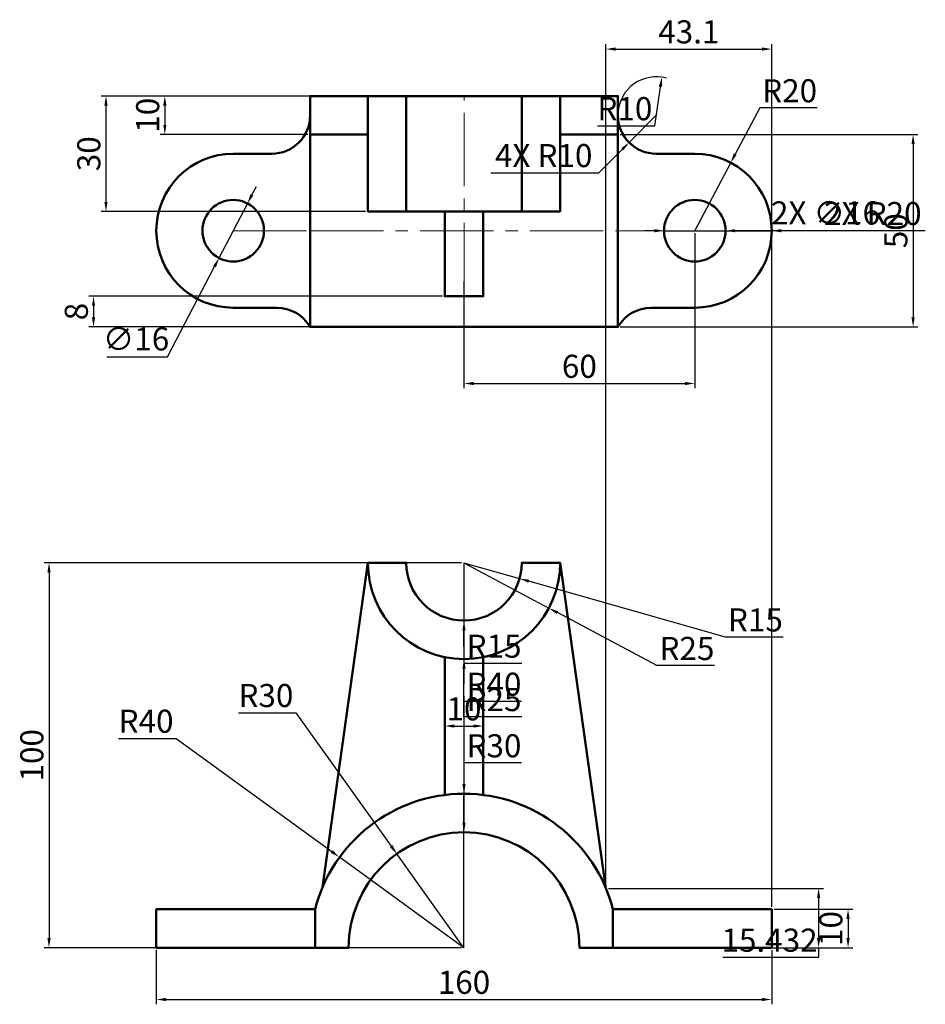
# Model space of a CAD drawing. Units: millimetres. Extents: x 81 to 317, y 95 to 351.
import ezdxf

# ---------------------------------------------------------------- set-up
doc = ezdxf.new("R2010")
doc.units = ezdxf.units.MM
doc.linetypes.add('CENTER2', pattern=[28.575, 19.05, -3.175, 3.175, -3.175])
for name, color, linetype, lineweight in [('M-CNTR', 1, 'CENTER2', 18), ('M-DIMS', 2, 'Continuous', 25), ('M-OUTL', 7, 'Continuous', 50)]:
    doc.layers.add(name, color=color, linetype=linetype, lineweight=lineweight)
doc.styles.get("Standard").update_dxf_attribs({"font": 'arial.ttf'})
doc.dimstyles.new('ISO-25', dxfattribs={"dimtxt": 6, "dimasz": 2.5, "dimexe": 1.25, "dimexo": 0.625, "dimtad": 1, "dimtoh": 1, "dimdec": 0, "dimtxsty": 'Standard', "dimcen": 2.5, "dimadec": 0, "dimazin": 0, "dimtfac": 1, "dimtdec": 0, "dimtmove": 0, "dimatfit": 3, "dimfxl": 1, "dimarcsym": 0})

# ---------------------------------------------------------------- blocks, each defined once
blk = doc.blocks.new('*D1')
at = {"layer": 'Defpoints', "color": 0, "transparency": 16777216}
for p in [(156.66, 331.08), (118.88, 321.08), (156.66, 321.08)]:
    blk.add_point(p, dxfattribs=at)
at = {"layer": 'M-DIMS', "color": 0, "lineweight": -2, "transparency": 16777216}
for p, q in [((156.04, 331.08), (117.63, 331.08)), ((118.88, 328.58), (118.88, 323.58)), ((156.04, 321.08), (117.63, 321.08))]:
    blk.add_line(p, q, dxfattribs=at)
at = {"layer": 'M-DIMS', "color": 0, "transparency": 16777216}
for points in [[(118.47, 328.58), (119.3, 328.58), (118.88, 331.08)], [(118.47, 323.58), (119.3, 323.58), (118.88, 321.08)]]:
    blk.add_solid(points, dxfattribs=at)
at = {"layer": 'M-DIMS', "color": 0, "transparency": 16777216, "insert": (115.2, 326.08), "char_height": 6, "attachment_point": 5, "rotation": 90}
blk.add_mtext('10', dxfattribs=at)
blk = doc.blocks.new('*D2')
at = {"layer": 'Defpoints', "color": 0, "transparency": 16777216}
for p in [(236.66, 321.08), (236.66, 271.08), (313.42, 271.08)]:
    blk.add_point(p, dxfattribs=at)
at = {"layer": 'M-DIMS', "color": 0, "lineweight": -2, "transparency": 16777216}
for p, q in [((237.29, 321.08), (314.67, 321.08)), ((313.42, 318.58), (313.42, 273.58)), ((237.29, 271.08), (314.67, 271.08))]:
    blk.add_line(p, q, dxfattribs=at)
at = {"layer": 'M-DIMS', "color": 0, "transparency": 16777216}
for points in [[(313, 318.58), (313.84, 318.58), (313.42, 321.08)], [(313, 273.58), (313.84, 273.58), (313.42, 271.08)]]:
    blk.add_solid(points, dxfattribs=at)
at = {"layer": 'M-DIMS', "color": 0, "transparency": 16777216, "insert": (309.73, 296.08), "char_height": 6, "attachment_point": 5, "rotation": 90}
blk.add_mtext('50', dxfattribs=at)
blk = doc.blocks.new('*D3')
at = {"layer": 'Defpoints', "color": 0, "transparency": 16777216}
for p in [(171.66, 331.08), (103.58, 301.08), (171.66, 301.08)]:
    blk.add_point(p, dxfattribs=at)
at = {"layer": 'M-DIMS', "color": 0, "lineweight": -2, "transparency": 16777216}
for p, q in [((171.04, 331.08), (102.33, 331.08)), ((103.58, 328.58), (103.58, 303.58)), ((171.04, 301.08), (102.33, 301.08))]:
    blk.add_line(p, q, dxfattribs=at)
at = {"layer": 'M-DIMS', "color": 0, "transparency": 16777216}
for points in [[(103.16, 328.58), (104, 328.58), (103.58, 331.08)], [(103.16, 303.58), (104, 303.58), (103.58, 301.08)]]:
    blk.add_solid(points, dxfattribs=at)
at = {"layer": 'M-DIMS', "color": 0, "transparency": 16777216, "insert": (99.89, 316.08), "char_height": 6, "attachment_point": 5, "rotation": 90}
blk.add_mtext('30', dxfattribs=at)
blk = doc.blocks.new('*D4')
at = {"layer": 'Defpoints', "color": 0, "transparency": 16777216}
for p in [(256.66, 296.08), (196.66, 283.5), (256.66, 256.39)]:
    blk.add_point(p, dxfattribs=at)
at = {"layer": 'M-DIMS', "color": 0, "lineweight": -2, "transparency": 16777216}
for p, q in [((256.66, 295.45), (256.66, 255.14)), ((196.66, 282.87), (196.66, 255.14)), ((199.16, 256.39), (254.16, 256.39))]:
    blk.add_line(p, q, dxfattribs=at)
at = {"layer": 'M-DIMS', "color": 0, "transparency": 16777216}
for points in [[(199.16, 256.81), (199.16, 255.98), (196.66, 256.39)], [(254.16, 256.81), (254.16, 255.98), (256.66, 256.39)]]:
    blk.add_solid(points, dxfattribs=at)
at = {"layer": 'M-DIMS', "color": 0, "transparency": 16777216, "insert": (226.66, 260.08), "char_height": 6, "attachment_point": 5}
blk.add_mtext('60', dxfattribs=at)
blk = doc.blocks.new('*D5')
at = {"layer": 'Defpoints', "color": 0, "transparency": 16777216}
for p in [(191.66, 279.08), (100.34, 271.08), (191.66, 271.08)]:
    blk.add_point(p, dxfattribs=at)
at = {"layer": 'M-DIMS', "color": 0, "lineweight": -2, "transparency": 16777216}
for p, q in [((191.04, 279.08), (99.09, 279.08)), ((100.34, 276.58), (100.34, 273.58)), ((191.04, 271.08), (99.09, 271.08))]:
    blk.add_line(p, q, dxfattribs=at)
at = {"layer": 'M-DIMS', "color": 0, "transparency": 16777216}
for points in [[(99.92, 276.58), (100.75, 276.58), (100.34, 279.08)], [(99.92, 273.58), (100.75, 273.58), (100.34, 271.08)]]:
    blk.add_solid(points, dxfattribs=at)
at = {"layer": 'M-DIMS', "color": 0, "transparency": 16777216, "insert": (96.65, 275.08), "char_height": 6, "attachment_point": 5, "rotation": 90}
blk.add_mtext('8', dxfattribs=at)
blk = doc.blocks.new('*D6')
at = {"layer": 'Defpoints', "color": 0, "transparency": 16777216}
for p in [(266.02, 313.76), (256.66, 296.08)]:
    blk.add_point(p, dxfattribs=at)
at = {"layer": 'M-DIMS', "color": 0, "lineweight": -2, "transparency": 16777216}
for p, q in [((273.54, 327.98), (267.19, 315.97)), ((288.48, 327.98), (273.54, 327.98)), ((256.66, 296.08), (266.02, 313.76))]:
    blk.add_line(p, q, dxfattribs=at)
at = {"layer": 'M-DIMS', "color": 0, "transparency": 16777216}
blk.add_solid([(266.82, 316.16), (267.55, 315.77), (266.02, 313.76)], dxfattribs=at)
at = {"layer": 'M-DIMS', "color": 0, "transparency": 16777216, "insert": (281.32, 331.67), "char_height": 6, "attachment_point": 5}
blk.add_mtext('R20', dxfattribs=at)
blk = doc.blocks.new('*D7')
at = {"layer": 'Defpoints', "color": 0, "transparency": 16777216}
for p in [(140.37, 303.17), (132.96, 288.99)]:
    blk.add_point(p, dxfattribs=at)
at = {"layer": 'M-DIMS', "color": 0, "lineweight": -2, "transparency": 16777216}
for p, q in [((141.52, 305.39), (142.68, 307.6)), ((140.37, 303.17), (132.96, 288.99)), ((119.58, 263.34), (131.81, 286.77)), ((103.84, 263.34), (119.58, 263.34))]:
    blk.add_line(p, q, dxfattribs=at)
at = {"layer": 'M-DIMS', "color": 0, "transparency": 16777216}
for points in [[(141.15, 305.58), (141.89, 305.19), (140.37, 303.17)], [(131.44, 286.96), (132.18, 286.58), (132.96, 288.99)]]:
    blk.add_solid(points, dxfattribs=at)
at = {"layer": 'M-DIMS', "color": 0, "transparency": 16777216, "insert": (111.4, 267.2), "char_height": 6, "attachment_point": 5}
blk.add_mtext('∅16', dxfattribs=at)
blk = doc.blocks.new('*D8')
at = {"layer": 'Defpoints', "color": 0, "transparency": 16777216}
for p in [(248.09, 335.98), (246.66, 326.08)]:
    blk.add_point(p, dxfattribs=at)
at = {"layer": 'M-DIMS', "color": 0, "lineweight": -2, "transparency": 16777216}
for p, q in [((246.27, 323.32), (247.73, 333.5)), ((231.33, 323.32), (246.27, 323.32))]:
    blk.add_line(p, q, dxfattribs=at)
blk.add_arc((246.66, 326.08), 10, 74.6697, 176.419, dxfattribs=at)
at = {"layer": 'M-DIMS', "color": 0, "transparency": 16777216}
blk.add_solid([(247.32, 333.56), (248.14, 333.44), (248.09, 335.98)], dxfattribs=at)
at = {"layer": 'M-DIMS', "color": 0, "transparency": 16777216, "insert": (238.49, 327.01), "char_height": 6, "attachment_point": 5}
blk.add_mtext('R10', dxfattribs=at)
blk = doc.blocks.new('*D9')
at = {"layer": 'Defpoints', "color": 0, "transparency": 16777216}
for p in [(196.66, 209.81), (88.77, 109.81), (196.66, 109.81)]:
    blk.add_point(p, dxfattribs=at)
at = {"layer": 'M-DIMS', "color": 0, "lineweight": -2, "transparency": 16777216}
for p, q in [((196.04, 209.81), (87.52, 209.81)), ((88.77, 207.31), (88.77, 112.31)), ((196.04, 109.81), (87.52, 109.81))]:
    blk.add_line(p, q, dxfattribs=at)
at = {"layer": 'M-DIMS', "color": 0, "transparency": 16777216}
for points in [[(88.35, 207.31), (89.19, 207.31), (88.77, 209.81)], [(88.35, 112.31), (89.19, 112.31), (88.77, 109.81)]]:
    blk.add_solid(points, dxfattribs=at)
at = {"layer": 'M-DIMS', "color": 0, "transparency": 16777216, "insert": (85.08, 159.81), "char_height": 6, "attachment_point": 5, "rotation": 90}
blk.add_mtext('100', dxfattribs=at)
blk = doc.blocks.new('*D10')
at = {"layer": 'Defpoints', "color": 0, "transparency": 16777216}
for p in [(191.66, 167.4), (201.66, 167.4), (201.66, 167.4)]:
    blk.add_point(p, dxfattribs=at)
at = {"layer": 'M-DIMS', "color": 0, "lineweight": -2, "transparency": 16777216}
for p, q in [((191.66, 168.03), (191.66, 168.65)), ((194.16, 167.4), (199.16, 167.4)), ((201.66, 168.03), (201.66, 168.65))]:
    blk.add_line(p, q, dxfattribs=at)
at = {"layer": 'M-DIMS', "color": 0, "transparency": 16777216}
for points in [[(194.16, 167.82), (194.16, 166.99), (191.66, 167.4)], [(199.16, 167.82), (199.16, 166.99), (201.66, 167.4)]]:
    blk.add_solid(points, dxfattribs=at)
at = {"layer": 'M-DIMS', "color": 0, "transparency": 16777216, "insert": (196.66, 171.09), "char_height": 6, "attachment_point": 5}
blk.add_mtext('10', dxfattribs=at)
blk = doc.blocks.new('*D11')
at = {"layer": 'Defpoints', "color": 0, "transparency": 16777216}
for p in [(276.66, 119.81), (276.66, 109.81), (296.51, 109.81)]:
    blk.add_point(p, dxfattribs=at)
at = {"layer": 'M-DIMS', "color": 0, "lineweight": -2, "transparency": 16777216}
for p, q in [((277.29, 119.81), (297.76, 119.81)), ((296.51, 117.31), (296.51, 112.31)), ((277.29, 109.81), (297.76, 109.81))]:
    blk.add_line(p, q, dxfattribs=at)
at = {"layer": 'M-DIMS', "color": 0, "transparency": 16777216}
for points in [[(296.09, 117.31), (296.93, 117.31), (296.51, 119.81)], [(296.09, 112.31), (296.93, 112.31), (296.51, 109.81)]]:
    blk.add_solid(points, dxfattribs=at)
at = {"layer": 'M-DIMS', "color": 0, "transparency": 16777216, "insert": (292.82, 114.81), "char_height": 6, "attachment_point": 5, "rotation": 90}
blk.add_mtext('10', dxfattribs=at)
blk = doc.blocks.new('*D12')
at = {"layer": 'Defpoints', "color": 0, "transparency": 16777216}
for p in [(196.66, 209.81), (218.73, 198.05)]:
    blk.add_point(p, dxfattribs=at)
at = {"layer": 'M-DIMS', "color": 0, "lineweight": -2, "transparency": 16777216}
for p, q in [((196.66, 209.81), (218.73, 198.05)), ((246.8, 183.1), (220.94, 196.88)), ((261.81, 183.1), (246.8, 183.1))]:
    blk.add_line(p, q, dxfattribs=at)
at = {"layer": 'M-DIMS', "color": 0, "transparency": 16777216}
blk.add_solid([(221.13, 197.25), (220.74, 196.51), (218.73, 198.05)], dxfattribs=at)
at = {"layer": 'M-DIMS', "color": 0, "transparency": 16777216, "insert": (254.62, 186.79), "char_height": 6, "attachment_point": 5}
blk.add_mtext('R25', dxfattribs=at)
blk = doc.blocks.new('*D13')
at = {"layer": 'Defpoints', "color": 0, "transparency": 16777216}
for p in [(196.66, 209.81), (211.09, 205.71)]:
    blk.add_point(p, dxfattribs=at)
at = {"layer": 'M-DIMS', "color": 0, "lineweight": -2, "transparency": 16777216}
for p, q in [((196.66, 209.81), (211.09, 205.71)), ((264.61, 190.51), (213.5, 205.03)), ((279.61, 190.51), (264.61, 190.51))]:
    blk.add_line(p, q, dxfattribs=at)
at = {"layer": 'M-DIMS', "color": 0, "transparency": 16777216}
blk.add_solid([(213.61, 205.43), (213.39, 204.63), (211.09, 205.71)], dxfattribs=at)
at = {"layer": 'M-DIMS', "color": 0, "transparency": 16777216, "insert": (272.42, 194.2), "char_height": 6, "attachment_point": 5}
blk.add_mtext('R15', dxfattribs=at)
blk = doc.blocks.new('*D14')
at = {"layer": 'Defpoints', "color": 0, "transparency": 16777216}
for p in [(116.66, 109.81), (276.66, 109.81), (276.66, 96.36)]:
    blk.add_point(p, dxfattribs=at)
at = {"layer": 'M-DIMS', "color": 0, "lineweight": -2, "transparency": 16777216}
for p, q in [((116.66, 109.18), (116.66, 95.11)), ((276.66, 109.18), (276.66, 95.11)), ((119.16, 96.36), (274.16, 96.36))]:
    blk.add_line(p, q, dxfattribs=at)
at = {"layer": 'M-DIMS', "color": 0, "transparency": 16777216}
for points in [[(119.16, 96.78), (119.16, 95.95), (116.66, 96.36)], [(274.16, 96.78), (274.16, 95.95), (276.66, 96.36)]]:
    blk.add_solid(points, dxfattribs=at)
at = {"layer": 'M-DIMS', "color": 0, "transparency": 16777216, "insert": (196.66, 100.05), "char_height": 6, "attachment_point": 5}
blk.add_mtext('160', dxfattribs=at)
blk = doc.blocks.new('*D15')
at = {"layer": 'Defpoints', "color": 0, "transparency": 16777216}
for p in [(164.3, 133.32), (196.66, 109.81)]:
    blk.add_point(p, dxfattribs=at)
at = {"layer": 'M-DIMS', "color": 0, "lineweight": -2, "transparency": 16777216}
for p, q in [((106.84, 164.2), (121.79, 164.2)), ((121.79, 164.2), (162.28, 134.79)), ((196.66, 109.81), (164.3, 133.32))]:
    blk.add_line(p, q, dxfattribs=at)
at = {"layer": 'M-DIMS', "color": 0, "transparency": 16777216}
blk.add_solid([(162.52, 135.12), (162.03, 134.45), (164.3, 133.32)], dxfattribs=at)
at = {"layer": 'M-DIMS', "color": 0, "transparency": 16777216, "insert": (114, 167.88), "char_height": 6, "attachment_point": 5}
blk.add_mtext('R40', dxfattribs=at)
blk = doc.blocks.new('*D16')
at = {"layer": 'Defpoints', "color": 0, "transparency": 16777216}
for p in [(179.2, 134.2), (196.66, 109.81)]:
    blk.add_point(p, dxfattribs=at)
at = {"layer": 'M-DIMS', "color": 0, "lineweight": -2, "transparency": 16777216}
for p, q in [((138, 170.87), (152.95, 170.87)), ((152.95, 170.87), (177.74, 136.23)), ((196.66, 109.81), (179.2, 134.2))]:
    blk.add_line(p, q, dxfattribs=at)
at = {"layer": 'M-DIMS', "color": 0, "transparency": 16777216}
blk.add_solid([(178.08, 136.48), (177.41, 135.99), (179.2, 134.2)], dxfattribs=at)
at = {"layer": 'M-DIMS', "color": 0, "transparency": 16777216, "insert": (145.16, 174.56), "char_height": 6, "attachment_point": 5}
blk.add_mtext('R30', dxfattribs=at)
blk = doc.blocks.new('*D17')
at = {"layer": 'Defpoints', "color": 0, "transparency": 16777216}
for p in [(276.66, 343.28), (233.57, 125.24), (276.66, 119.81)]:
    blk.add_point(p, dxfattribs=at)
at = {"layer": 'M-DIMS', "color": 0, "lineweight": -2, "transparency": 16777216}
for p, q in [((233.57, 125.87), (233.57, 344.53)), ((236.07, 343.28), (274.16, 343.28)), ((276.66, 120.43), (276.66, 344.53))]:
    blk.add_line(p, q, dxfattribs=at)
at = {"layer": 'M-DIMS', "color": 0, "transparency": 16777216}
for points in [[(236.07, 343.7), (236.07, 342.86), (233.57, 343.28)], [(274.16, 343.7), (274.16, 342.86), (276.66, 343.28)]]:
    blk.add_solid(points, dxfattribs=at)
at = {"layer": 'M-DIMS', "color": 0, "transparency": 16777216, "insert": (255.12, 346.97), "char_height": 6, "attachment_point": 5}
blk.add_mtext('43.1', dxfattribs=at)
blk = doc.blocks.new('*D18')
at = {"layer": 'Defpoints', "color": 0, "transparency": 16777216}
for p in [(233.57, 125.24), (235.39, 109.81), (288.86, 109.81)]:
    blk.add_point(p, dxfattribs=at)
at = {"layer": 'M-DIMS', "color": 0, "lineweight": -2, "transparency": 16777216}
for p, q in [((234.19, 125.24), (290.11, 125.24)), ((288.86, 122.74), (288.86, 112.31)), ((236.02, 109.81), (290.11, 109.81)), ((288.86, 109.81), (288.86, 107.31)), ((288.86, 107.31), (263.96, 107.31))]:
    blk.add_line(p, q, dxfattribs=at)
at = {"layer": 'M-DIMS', "color": 0, "transparency": 16777216}
for points in [[(288.45, 122.74), (289.28, 122.74), (288.86, 125.24)], [(288.45, 112.31), (289.28, 112.31), (288.86, 109.81)]]:
    blk.add_solid(points, dxfattribs=at)
at = {"layer": 'M-DIMS', "color": 0, "transparency": 16777216, "insert": (276.1, 111), "char_height": 6, "attachment_point": 5}
blk.add_mtext('15.432', dxfattribs=at)
blk = doc.blocks.new('*D19')
at = {"layer": 'Defpoints', "color": 0, "transparency": 16777216}
for p in [(196.66, 149.81), (196.66, 109.81)]:
    blk.add_point(p, dxfattribs=at)
at = {"layer": 'M-DIMS', "color": 0, "lineweight": -2, "transparency": 16777216}
for p, q in [((211.61, 173.81), (196.66, 173.81)), ((196.66, 173.81), (196.66, 152.31)), ((196.66, 109.81), (196.66, 149.81))]:
    blk.add_line(p, q, dxfattribs=at)
at = {"layer": 'M-DIMS', "color": 0, "transparency": 16777216}
blk.add_solid([(196.25, 152.31), (197.08, 152.31), (196.66, 149.81)], dxfattribs=at)
at = {"layer": 'M-DIMS', "color": 0, "transparency": 16777216, "insert": (204.45, 177.5), "char_height": 6, "attachment_point": 5}
blk.add_mtext('R40', dxfattribs=at)
blk = doc.blocks.new('*D20')
at = {"layer": 'Defpoints', "color": 0, "transparency": 16777216}
for p in [(196.66, 139.81), (196.66, 109.81)]:
    blk.add_point(p, dxfattribs=at)
at = {"layer": 'M-DIMS', "color": 0, "lineweight": -2, "transparency": 16777216}
for p, q in [((211.61, 157.81), (196.66, 157.81)), ((196.66, 157.81), (196.66, 142.31)), ((196.66, 109.81), (196.66, 139.81))]:
    blk.add_line(p, q, dxfattribs=at)
at = {"layer": 'M-DIMS', "color": 0, "transparency": 16777216}
blk.add_solid([(196.25, 142.31), (197.08, 142.31), (196.66, 139.81)], dxfattribs=at)
at = {"layer": 'M-DIMS', "color": 0, "transparency": 16777216, "insert": (204.45, 161.5), "char_height": 6, "attachment_point": 5}
blk.add_mtext('R30', dxfattribs=at)
blk = doc.blocks.new('*D21')
at = {"layer": 'Defpoints', "color": 0, "transparency": 16777216}
for p in [(196.66, 209.81), (196.66, 184.81)]:
    blk.add_point(p, dxfattribs=at)
at = {"layer": 'M-DIMS', "color": 0, "lineweight": -2, "transparency": 16777216}
for p, q in [((196.66, 209.81), (196.66, 184.81)), ((196.66, 169.81), (196.66, 182.31)), ((211.67, 169.81), (196.66, 169.81))]:
    blk.add_line(p, q, dxfattribs=at)
at = {"layer": 'M-DIMS', "color": 0, "transparency": 16777216}
blk.add_solid([(197.08, 182.31), (196.25, 182.31), (196.66, 184.81)], dxfattribs=at)
at = {"layer": 'M-DIMS', "color": 0, "transparency": 16777216, "insert": (204.48, 173.5), "char_height": 6, "attachment_point": 5}
blk.add_mtext('R25', dxfattribs=at)
blk = doc.blocks.new('*D22')
at = {"layer": 'Defpoints', "color": 0, "transparency": 16777216}
for p in [(196.66, 209.81), (196.66, 194.81)]:
    blk.add_point(p, dxfattribs=at)
at = {"layer": 'M-DIMS', "color": 0, "lineweight": -2, "transparency": 16777216}
for p, q in [((196.66, 209.81), (196.66, 194.81)), ((196.67, 183.68), (196.66, 192.31)), ((211.67, 183.68), (196.67, 183.68))]:
    blk.add_line(p, q, dxfattribs=at)
at = {"layer": 'M-DIMS', "color": 0, "transparency": 16777216}
blk.add_solid([(197.08, 192.31), (196.25, 192.31), (196.66, 194.81)], dxfattribs=at)
at = {"layer": 'M-DIMS', "color": 0, "transparency": 16777216, "insert": (204.48, 187.37), "char_height": 6, "attachment_point": 5}
blk.add_mtext('R15', dxfattribs=at)
blk = doc.blocks.new('*D23')
at = {"layer": 'Defpoints', "color": 0, "transparency": 16777216}
for p in [(256.66, 296.08), (276.66, 296.08)]:
    blk.add_point(p, dxfattribs=at)
at = {"layer": 'M-DIMS', "color": 0, "lineweight": -2, "transparency": 16777216}
for p, q in [((256.66, 296.08), (276.66, 296.08)), ((288.66, 296.08), (279.16, 296.08)), ((316.6, 296.08), (288.66, 296.08))]:
    blk.add_line(p, q, dxfattribs=at)
at = {"layer": 'M-DIMS', "color": 0, "transparency": 16777216}
blk.add_solid([(279.16, 296.5), (279.16, 295.66), (276.66, 296.08)], dxfattribs=at)
at = {"layer": 'M-DIMS', "color": 0, "transparency": 16777216, "insert": (302.95, 299.77), "char_height": 6, "attachment_point": 5}
blk.add_mtext('2X R20', dxfattribs=at)
blk = doc.blocks.new('*D24')
at = {"layer": 'Defpoints', "color": 0, "transparency": 16777216}
for p in [(246.66, 326.08), (239.59, 319.01)]:
    blk.add_point(p, dxfattribs=at)
at = {"layer": 'M-DIMS', "color": 0, "lineweight": -2, "transparency": 16777216}
for p, q in [((246.66, 326.08), (239.59, 319.01)), ((231.73, 311.14), (237.83, 317.24)), ((203.65, 311.14), (231.73, 311.14))]:
    blk.add_line(p, q, dxfattribs=at)
at = {"layer": 'M-DIMS', "color": 0, "transparency": 16777216}
blk.add_solid([(237.53, 317.53), (238.12, 316.95), (239.59, 319.01)], dxfattribs=at)
at = {"layer": 'M-DIMS', "color": 0, "transparency": 16777216, "insert": (217.38, 314.83), "char_height": 6, "attachment_point": 5}
blk.add_mtext('4X R10', dxfattribs=at)
blk = doc.blocks.new('*D25')
at = {"layer": 'Defpoints', "color": 0, "transparency": 16777216}
for p in [(248.66, 296.08), (264.66, 296.08)]:
    blk.add_point(p, dxfattribs=at)
at = {"layer": 'M-DIMS', "color": 0, "lineweight": -2, "transparency": 16777216}
for p, q in [((246.16, 296.08), (243.66, 296.08)), ((248.66, 296.08), (264.66, 296.08)), ((276.13, 296.08), (267.16, 296.08)), ((304.55, 296.08), (276.13, 296.08))]:
    blk.add_line(p, q, dxfattribs=at)
at = {"layer": 'M-DIMS', "color": 0, "transparency": 16777216}
for points in [[(246.16, 296.5), (246.16, 295.66), (248.66, 296.08)], [(267.16, 296.5), (267.16, 295.66), (264.66, 296.08)]]:
    blk.add_solid(points, dxfattribs=at)
at = {"layer": 'M-DIMS', "color": 0, "transparency": 16777216, "insert": (290.65, 299.94), "char_height": 6, "attachment_point": 5}
blk.add_mtext('2X ∅16', dxfattribs=at)

msp = doc.modelspace()

# ---------------------------------------------------------------- linework, layer by layer
at = {"layer": 'M-CNTR'}
for p, q in [((196.6648, 279.0792), (196.6648, 331.0792)), ((196.6648, 149.8091), (196.6648, 184.8091))]:
    msp.add_line(p, q, dxfattribs=at)
msp.add_lwpolyline([(136.6648, 296.0792), (156.6648, 296.0792), (236.6648, 296.0792), (256.6648, 296.0792)], dxfattribs=at)
at = {"layer": 'M-OUTL'}
for p, q in [((181.6648, 301.0792), (181.6648, 331.0792)), ((211.6648, 301.0792), (211.6648, 331.0792)), ((156.6648, 321.0792), (171.6648, 321.0792)), ((221.6648, 321.0792), (236.6648, 321.0792)), ((236.6648, 271.0792), (156.6648, 271.0792)), ((191.6648, 149.4954), (191.6648, 185.3142)), ((201.6648, 149.4954), (201.6648, 185.3142))]:
    msp.add_line(p, q, dxfattribs=at)
for points in [[(236.6648, 326.0792, 0.41421356), (246.6648, 316.0792), (256.6648, 316.0792, -1), (256.6648, 276.0792), (245.3251, 276.0792, 0.26794919), (236.6648, 271.0792), (236.6648, 324.0792), (236.6648, 331.0792), (156.6648, 331.0792), (156.6648, 271.0792, 0.26794919), (148.0046, 276.0792), (136.6648, 276.0792, -1), (136.6648, 316.0792), (146.6648, 316.0792, 0.41421356), (156.6648, 326.0792)], [(159.8858, 125.535), (171.6648, 209.8091), (181.6648, 209.8091, 1), (211.6648, 209.8091), (221.6648, 209.8091), (233.5681, 125.2412)], [(157.935, 109.8091), (157.935, 119.8091), (116.6648, 119.8091), (116.6648, 109.8091), (156.6648, 109.8091), (166.6648, 109.8091, -1), (226.6648, 109.8091), (236.6648, 109.8091), (276.6648, 109.8091), (276.6648, 119.8091), (235.3946, 119.8091), (235.3946, 109.8091)]]:
    msp.add_lwpolyline(points, format="xyb", dxfattribs=at)
for points in [[(171.6648, 331.0792), (171.6648, 301.0792), (221.6648, 301.0792), (221.6648, 331.0792)], [(201.6648, 301.0792), (201.6648, 279.0792), (191.6648, 279.0792), (191.6648, 301.0792)]]:
    msp.add_lwpolyline(points, dxfattribs=at)
for centre in [(136.6648, 296.0792), (256.6648, 296.0792)]:
    msp.add_circle(centre, 8, dxfattribs=at)
for centre, radius, start, end in [((196.6648, 209.8091), 25, 180, 0), ((196.6648, 109.8091), 40, 14.477512, 165.522488)]:
    msp.add_arc(centre, radius, start, end, dxfattribs=at)

# ---------------------------------------------------------------- dimensions: what is measured, and where the dimension line sits
at = {"layer": 'M-DIMS'}
for base, p1, p2, override, picture, middle in [((276.6648, 343.2792), (233.5681, 125.2412), (276.6648, 119.8091), {"dimdec": 1, "dimlfac": 1, "dimrnd": 0, "dimzin": 0, "dimdsep": 46, "dimlunit": 2}, '*D17', (255.1164, 346.9696)), ((256.6648, 256.3919), (196.6648, 283.4983), (256.6648, 296.0792), {"dimclrd": 0, "dimclre": 0, "dimclrt": 0}, '*D4', (226.6648, 260.0804)), ((201.6648, 167.4048), (191.6648, 167.4048), (201.6648, 167.4048), {"dimclrd": 0, "dimclre": 0, "dimclrt": 0}, '*D10', (196.6648, 171.0932)), ((276.6648, 96.3645), (116.6648, 109.8091), (276.6648, 109.8091), {"dimclrd": 0, "dimclre": 0, "dimclrt": 0}, '*D14', (196.6648, 100.0529))]:
    dim = msp.add_linear_dim(base=base, p1=p1, p2=p2, dimstyle='ISO-25', override=override, dxfattribs=at)
    dim.commit()
    dim.dimension.update_dxf_attribs({"geometry": picture, "text_midpoint": middle})
for center, mpoint, override, picture, middle in [((246.6648, 326.0792), (248.0856, 335.9777), {"dimclrd": 0, "dimclre": 0, "dimclrt": 0}, '*D8', (238.4861, 323.3241)), ((256.6648, 296.0792), (266.0164, 313.7582), {"dimclrd": 0, "dimclre": 0, "dimclrt": 0}, '*D6', (281.3228, 327.9806)), ((196.6648, 209.8091), (196.665, 184.8091), {"dimdec": 0, "dimlfac": 1, "dimrnd": 0, "dimzin": 0, "dimdsep": 46, "dimlunit": 2}, '*D21', (204.4811, 169.8091)), ((196.6648, 209.8091), (218.7289, 198.0543), {"dimclrd": 0, "dimclre": 0, "dimclrt": 0}, '*D12', (254.616, 183.0993)), ((196.6648, 209.8091), (211.0941, 205.7109), {"dimclrd": 0, "dimclre": 0, "dimclrt": 0}, '*D13', (272.4222, 190.5125)), ((196.6648, 109.8091), (196.665, 149.8091), {"dimdec": 0, "dimlfac": 1, "dimrnd": 0, "dimzin": 0, "dimdsep": 46, "dimlunit": 2}, '*D19', (204.4484, 173.8091)), ((196.6648, 109.8091), (179.1998, 134.2012), {"dimclrd": 0, "dimclre": 0, "dimclrt": 0}, '*D16', (145.1632, 170.8674)), ((196.6648, 109.8091), (164.3007, 133.3159), {"dimclrd": 0, "dimclre": 0, "dimclrt": 0}, '*D15', (114.0024, 164.1955)), ((196.6648, 109.8091), (196.665, 139.8091), {"dimdec": 0, "dimlfac": 1, "dimrnd": 0, "dimzin": 0, "dimdsep": 46, "dimlunit": 2}, '*D20', (204.4484, 157.8091))]:
    dim = msp.add_radius_dim(center=center, mpoint=mpoint, dimstyle='ISO-25', override=override, dxfattribs=at)
    dim.commit()
    dim.dimension.update_dxf_attribs({"geometry": picture, "text_midpoint": middle, "dimtype": 164})
for base, p1, p2, override, picture, middle in [((103.5813, 301.0792), (171.6648, 331.0792), (171.6648, 301.0792), {"dimclrd": 0, "dimclre": 0, "dimclrt": 0}, '*D3', (99.8908, 316.0792)), ((118.8845, 321.0792), (156.6648, 331.0792), (156.6648, 321.0792), {"dimclrd": 0, "dimclre": 0, "dimclrt": 0}, '*D1', (115.196, 326.0792)), ((313.4207, 271.0792), (236.6648, 321.0792), (236.6648, 271.0792), {"dimclrd": 0, "dimclre": 0, "dimclrt": 0}, '*D2', (309.7322, 296.0792)), ((100.3351, 271.0792), (191.6648, 279.0792), (191.6648, 271.0792), {"dimclrd": 0, "dimclre": 0, "dimclrt": 0}, '*D5', (96.6467, 275.0792)), ((88.77, 109.8091), (196.6648, 209.8091), (196.6648, 109.8091), {"dimclrd": 0, "dimclre": 0, "dimclrt": 0}, '*D9', (85.0815, 159.8091)), ((288.8648, 109.8091), (233.5681, 125.2412), (235.3946, 109.8091), {"dimdec": 3, "dimlfac": 1, "dimrnd": 0, "dimzin": 0, "dimdsep": 46, "dimlunit": 2}, '*D18', (276.0986, 110.9996)), ((296.509, 109.8091), (276.6648, 119.8091), (276.6648, 109.8091), {"dimclrd": 0, "dimclre": 0, "dimclrt": 0}, '*D11', (292.8205, 114.8091))]:
    dim = msp.add_linear_dim(base=base, p1=p1, p2=p2, angle=90, dimstyle='ISO-25', override=override, dxfattribs=at)
    dim.commit()
    dim.dimension.update_dxf_attribs({"geometry": picture, "text_midpoint": middle})
dim = msp.add_radius_dim(center=(246.6648, 326.0792), mpoint=(239.5939, 319.0079), text='4X <>', dimstyle='ISO-25', override={"dimdec": 0, "dimlfac": 1, "dimrnd": 0, "dimzin": 0, "dimdsep": 46, "dimlunit": 2}, dxfattribs=at)
dim.commit()
dim.dimension.update_dxf_attribs({"geometry": '*D24', "text_midpoint": (217.3761, 314.8283)})
dim = msp.add_diameter_dim_2p(p1=(140.3661, 303.1714), p2=(132.9635, 288.9869), dimstyle='ISO-25', override={"dimclrd": 0, "dimclre": 0, "dimclrt": 0}, dxfattribs=at)
dim.commit()
dim.dimension.update_dxf_attribs({"geometry": '*D7', "text_midpoint": (111.3957, 263.3423), "dimtype": 163})
dim = msp.add_diameter_dim_2p(p1=(248.6648, 296.0793), p2=(264.6648, 296.079), text='2X <>', dimstyle='ISO-25', override={"dimdec": 0, "dimlfac": 1, "dimrnd": 0, "dimzin": 0, "dimdsep": 46, "dimlunit": 2}, dxfattribs=at)
dim.commit()
dim.dimension.update_dxf_attribs({"geometry": '*D25', "text_midpoint": (276.1273, 296.0788), "dimtype": 163})
dim = msp.add_radius_dim(center=(256.6648, 296.0792), mpoint=(276.6648, 296.079), text='2X <>', dimstyle='ISO-25', override={"dimdec": 0, "dimlfac": 1, "dimrnd": 0, "dimzin": 0, "dimdsep": 46, "dimlunit": 2}, dxfattribs=at)
dim.commit()
dim.dimension.update_dxf_attribs({"geometry": '*D23', "text_midpoint": (288.6648, 296.0789), "dimtype": 164})
dim = msp.add_radius_dim(center=(196.6648, 209.8091), mpoint=(196.665, 194.8091), dimstyle='ISO-25', override={"dimdec": 0, "dimlfac": 1, "dimrnd": 0, "dimzin": 0, "dimdsep": 46, "dimlunit": 2}, dxfattribs=at)
dim.commit()
dim.dimension.update_dxf_attribs({"geometry": '*D22', "text_midpoint": (204.4811, 187.3707)})

doc.saveas('drawing.dxf')
